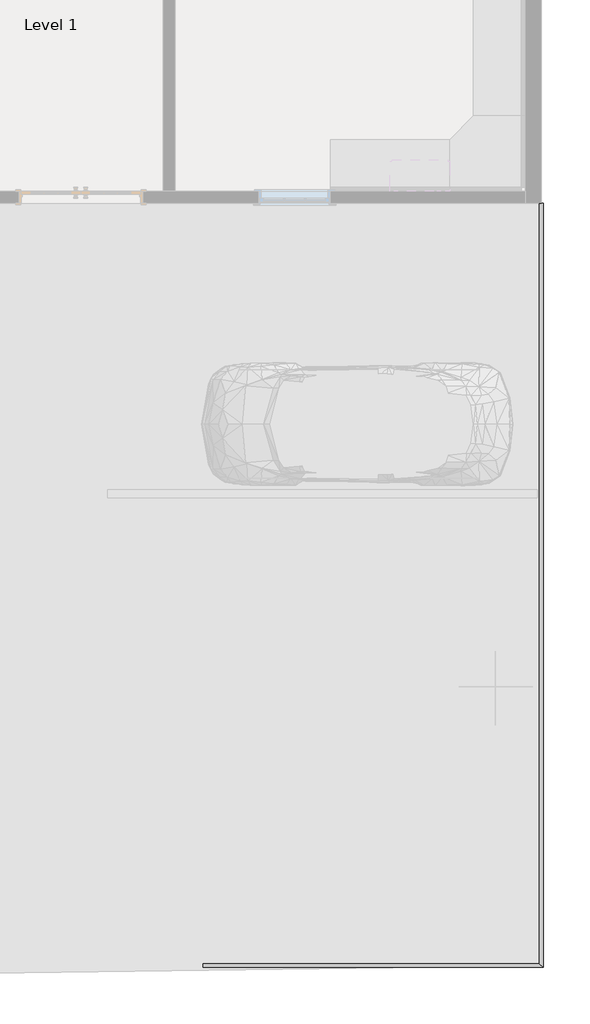
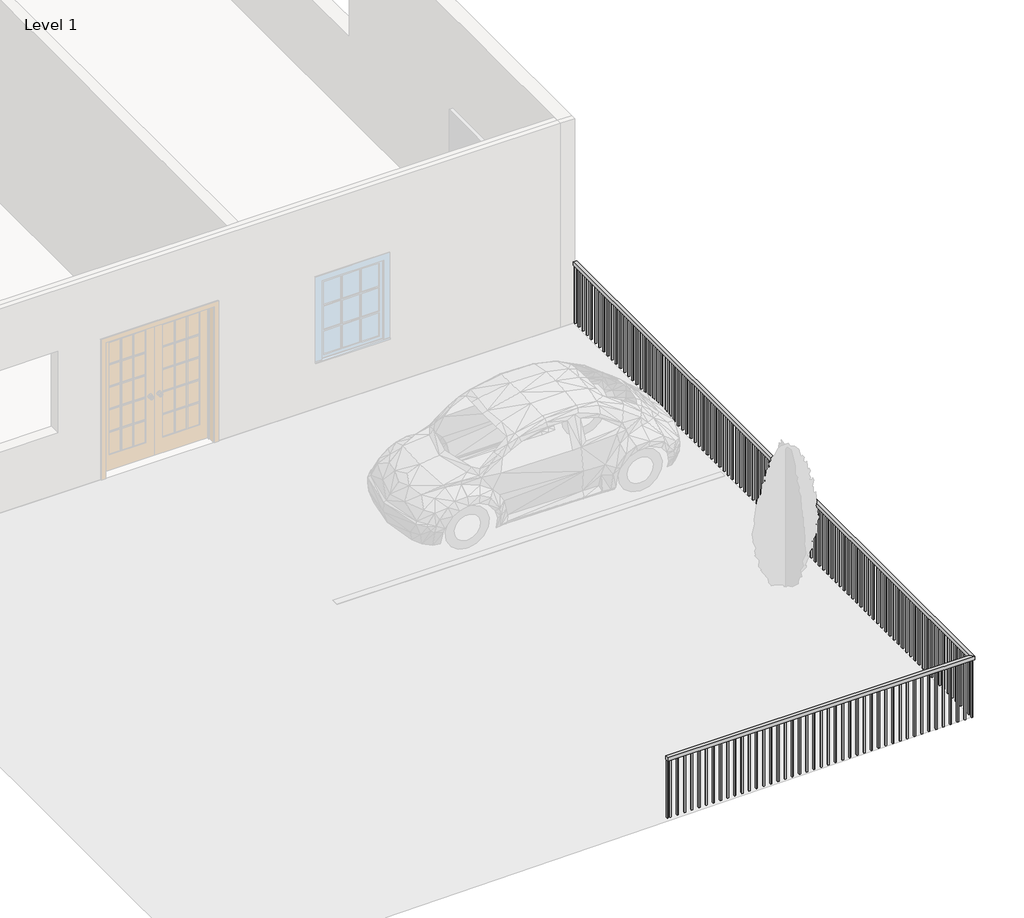
# One storey, part 3 of 5: 1 railing.
"""IFC4 building model written with IfcOpenShell, lengths in millimetres."""

from ifc_helpers import new_model, si_unit, origin, origin_with_axes, place, context, project, spatial, polyline, outline, extrude, faceted_brep, element, save

model = new_model("IFC4")

# Units and contexts
model_context = context("Model", 3, world=origin())
ifc_project = project(units=[si_unit("LENGTHUNIT", "METRE", prefix="MILLI")], contexts=[model_context])

# Site, building, storey
site = spatial("IfcSite", under=ifc_project)
building = spatial("IfcBuilding", under=site)
storey = spatial("IfcBuildingStorey", under=building, Name="Level 1", Elevation=0.0)

# Railing
placement = place(None, origin())
element("IfcRailing", 1, ObjectType="Handrail - Rectangular", at=placement, inside=storey, context=model_context, shape_type="SolidModel", body=[
    faceted_brep([(1884.1829734, -2473.4076646, 914.4), (1884.1829734, -2473.4076646, 863.6), (1833.3829734, -2473.4076646, 863.6), (1833.3829734, -2473.4076646, 914.4), (1884.1829734, -12227.0076646, 914.4), (1884.1829734, -12227.0076646, 863.6), (1833.3829734, -12176.2076646, 863.6), (1833.3829734, -12176.2076646, 914.4), (-2459.2170266, -12227.0076646, 914.4), (-2459.2170266, -12176.2076646, 914.4), (-2459.2170266, -12176.2076646, 863.6), (-2459.2170266, -12227.0076646, 863.6)], [[[0, 1, 2, 3]], [[1, 0, 4, 5]], [[2, 1, 5, 6]], [[3, 2, 6, 7]], [[0, 3, 7, 4]], [[8, 9, 10, 11]], [[5, 4, 8, 11]], [[6, 5, 11, 10]], [[7, 6, 10, 9]], [[4, 7, 9, 8]]]),
    extrude(outline(polyline([(-2398.8920266, -12192.0826646), (-2398.8920266, -12211.1326646), (-2417.9420266, -12211.1326646), (-2417.9420266, -12192.0826646), (-2398.8920266, -12192.0826646)])), origin_with_axes(), (0.0, 0.0, 1.0), 863.6),
    extrude(outline(polyline([(-2297.2920266, -12192.0826646), (-2297.2920266, -12211.1326646), (-2316.3420266, -12211.1326646), (-2316.3420266, -12192.0826646), (-2297.2920266, -12192.0826646)])), origin_with_axes(), (0.0, 0.0, 1.0), 863.6),
    extrude(outline(polyline([(-2195.6920266, -12192.0826646), (-2195.6920266, -12211.1326646), (-2214.7420266, -12211.1326646), (-2214.7420266, -12192.0826646), (-2195.6920266, -12192.0826646)])), origin_with_axes(), (0.0, 0.0, 1.0), 863.6),
    extrude(outline(polyline([(-2094.0920266, -12192.0826646), (-2094.0920266, -12211.1326646), (-2113.1420266, -12211.1326646), (-2113.1420266, -12192.0826646), (-2094.0920266, -12192.0826646)])), origin_with_axes(), (0.0, 0.0, 1.0), 863.6),
    extrude(outline(polyline([(-1992.4920266, -12192.0826646), (-1992.4920266, -12211.1326646), (-2011.5420266, -12211.1326646), (-2011.5420266, -12192.0826646), (-1992.4920266, -12192.0826646)])), origin_with_axes(), (0.0, 0.0, 1.0), 863.6),
    extrude(outline(polyline([(-1890.8920266, -12192.0826646), (-1890.8920266, -12211.1326646), (-1909.9420266, -12211.1326646), (-1909.9420266, -12192.0826646), (-1890.8920266, -12192.0826646)])), origin_with_axes(), (0.0, 0.0, 1.0), 863.6),
    extrude(outline(polyline([(-1789.2920266, -12192.0826646), (-1789.2920266, -12211.1326646), (-1808.3420266, -12211.1326646), (-1808.3420266, -12192.0826646), (-1789.2920266, -12192.0826646)])), origin_with_axes(), (0.0, 0.0, 1.0), 863.6),
    extrude(outline(polyline([(-1687.6920266, -12192.0826646), (-1687.6920266, -12211.1326646), (-1706.7420266, -12211.1326646), (-1706.7420266, -12192.0826646), (-1687.6920266, -12192.0826646)])), origin_with_axes(), (0.0, 0.0, 1.0), 863.6),
    extrude(outline(polyline([(-1586.0920266, -12192.0826646), (-1586.0920266, -12211.1326646), (-1605.1420266, -12211.1326646), (-1605.1420266, -12192.0826646), (-1586.0920266, -12192.0826646)])), origin_with_axes(), (0.0, 0.0, 1.0), 863.6),
    extrude(outline(polyline([(-1484.4920266, -12192.0826646), (-1484.4920266, -12211.1326646), (-1503.5420266, -12211.1326646), (-1503.5420266, -12192.0826646), (-1484.4920266, -12192.0826646)])), origin_with_axes(), (0.0, 0.0, 1.0), 863.6),
    extrude(outline(polyline([(-1382.8920266, -12192.0826646), (-1382.8920266, -12211.1326646), (-1401.9420266, -12211.1326646), (-1401.9420266, -12192.0826646), (-1382.8920266, -12192.0826646)])), origin_with_axes(), (0.0, 0.0, 1.0), 863.6),
    extrude(outline(polyline([(-1281.2920266, -12192.0826646), (-1281.2920266, -12211.1326646), (-1300.3420266, -12211.1326646), (-1300.3420266, -12192.0826646), (-1281.2920266, -12192.0826646)])), origin_with_axes(), (0.0, 0.0, 1.0), 863.6),
    extrude(outline(polyline([(-1179.6920266, -12192.0826646), (-1179.6920266, -12211.1326646), (-1198.7420266, -12211.1326646), (-1198.7420266, -12192.0826646), (-1179.6920266, -12192.0826646)])), origin_with_axes(), (0.0, 0.0, 1.0), 863.6),
    extrude(outline(polyline([(-1078.0920266, -12192.0826646), (-1078.0920266, -12211.1326646), (-1097.1420266, -12211.1326646), (-1097.1420266, -12192.0826646), (-1078.0920266, -12192.0826646)])), origin_with_axes(), (0.0, 0.0, 1.0), 863.6),
    extrude(outline(polyline([(-976.4920266, -12192.0826646), (-976.4920266, -12211.1326646), (-995.5420266, -12211.1326646), (-995.5420266, -12192.0826646), (-976.4920266, -12192.0826646)])), origin_with_axes(), (0.0, 0.0, 1.0), 863.6),
    extrude(outline(polyline([(-874.8920266, -12192.0826646), (-874.8920266, -12211.1326646), (-893.9420266, -12211.1326646), (-893.9420266, -12192.0826646), (-874.8920266, -12192.0826646)])), origin_with_axes(), (0.0, 0.0, 1.0), 863.6),
    extrude(outline(polyline([(-773.2920266, -12192.0826646), (-773.2920266, -12211.1326646), (-792.3420266, -12211.1326646), (-792.3420266, -12192.0826646), (-773.2920266, -12192.0826646)])), origin_with_axes(), (0.0, 0.0, 1.0), 863.6),
    extrude(outline(polyline([(-671.6920266, -12192.0826646), (-671.6920266, -12211.1326646), (-690.7420266, -12211.1326646), (-690.7420266, -12192.0826646), (-671.6920266, -12192.0826646)])), origin_with_axes(), (0.0, 0.0, 1.0), 863.6),
    extrude(outline(polyline([(-570.0920266, -12192.0826646), (-570.0920266, -12211.1326646), (-589.1420266, -12211.1326646), (-589.1420266, -12192.0826646), (-570.0920266, -12192.0826646)])), origin_with_axes(), (0.0, 0.0, 1.0), 863.6),
    extrude(outline(polyline([(-468.4920266, -12192.0826646), (-468.4920266, -12211.1326646), (-487.5420266, -12211.1326646), (-487.5420266, -12192.0826646), (-468.4920266, -12192.0826646)])), origin_with_axes(), (0.0, 0.0, 1.0), 863.6),
    extrude(outline(polyline([(-366.8920266, -12192.0826646), (-366.8920266, -12211.1326646), (-385.9420266, -12211.1326646), (-385.9420266, -12192.0826646), (-366.8920266, -12192.0826646)])), origin_with_axes(), (0.0, 0.0, 1.0), 863.6),
    extrude(outline(polyline([(-265.2920266, -12192.0826646), (-265.2920266, -12211.1326646), (-284.3420266, -12211.1326646), (-284.3420266, -12192.0826646), (-265.2920266, -12192.0826646)])), origin_with_axes(), (0.0, 0.0, 1.0), 863.6),
    extrude(outline(polyline([(-163.6920266, -12192.0826646), (-163.6920266, -12211.1326646), (-182.7420266, -12211.1326646), (-182.7420266, -12192.0826646), (-163.6920266, -12192.0826646)])), origin_with_axes(), (0.0, 0.0, 1.0), 863.6),
    extrude(outline(polyline([(-62.0920266, -12192.0826646), (-62.0920266, -12211.1326646), (-81.1420266, -12211.1326646), (-81.1420266, -12192.0826646), (-62.0920266, -12192.0826646)])), origin_with_axes(), (0.0, 0.0, 1.0), 863.6),
    extrude(outline(polyline([(39.5079734, -12192.0826646), (39.5079734, -12211.1326646), (20.4579734, -12211.1326646), (20.4579734, -12192.0826646), (39.5079734, -12192.0826646)])), origin_with_axes(), (0.0, 0.0, 1.0), 863.6),
    extrude(outline(polyline([(141.1079734, -12192.0826646), (141.1079734, -12211.1326646), (122.0579734, -12211.1326646), (122.0579734, -12192.0826646), (141.1079734, -12192.0826646)])), origin_with_axes(), (0.0, 0.0, 1.0), 863.6),
    extrude(outline(polyline([(242.7079734, -12192.0826646), (242.7079734, -12211.1326646), (223.6579734, -12211.1326646), (223.6579734, -12192.0826646), (242.7079734, -12192.0826646)])), origin_with_axes(), (0.0, 0.0, 1.0), 863.6),
    extrude(outline(polyline([(344.3079734, -12192.0826646), (344.3079734, -12211.1326646), (325.2579734, -12211.1326646), (325.2579734, -12192.0826646), (344.3079734, -12192.0826646)])), origin_with_axes(), (0.0, 0.0, 1.0), 863.6),
    extrude(outline(polyline([(445.9079734, -12192.0826646), (445.9079734, -12211.1326646), (426.8579734, -12211.1326646), (426.8579734, -12192.0826646), (445.9079734, -12192.0826646)])), origin_with_axes(), (0.0, 0.0, 1.0), 863.6),
    extrude(outline(polyline([(547.5079734, -12192.0826646), (547.5079734, -12211.1326646), (528.4579734, -12211.1326646), (528.4579734, -12192.0826646), (547.5079734, -12192.0826646)])), origin_with_axes(), (0.0, 0.0, 1.0), 863.6),
    extrude(outline(polyline([(649.1079734, -12192.0826646), (649.1079734, -12211.1326646), (630.0579734, -12211.1326646), (630.0579734, -12192.0826646), (649.1079734, -12192.0826646)])), origin_with_axes(), (0.0, 0.0, 1.0), 863.6),
    extrude(outline(polyline([(750.7079734, -12192.0826646), (750.7079734, -12211.1326646), (731.6579734, -12211.1326646), (731.6579734, -12192.0826646), (750.7079734, -12192.0826646)])), origin_with_axes(), (0.0, 0.0, 1.0), 863.6),
    extrude(outline(polyline([(852.3079734, -12192.0826646), (852.3079734, -12211.1326646), (833.2579734, -12211.1326646), (833.2579734, -12192.0826646), (852.3079734, -12192.0826646)])), origin_with_axes(), (0.0, 0.0, 1.0), 863.6),
    extrude(outline(polyline([(953.9079734, -12192.0826646), (953.9079734, -12211.1326646), (934.8579734, -12211.1326646), (934.8579734, -12192.0826646), (953.9079734, -12192.0826646)])), origin_with_axes(), (0.0, 0.0, 1.0), 863.6),
    extrude(outline(polyline([(1055.5079734, -12192.0826646), (1055.5079734, -12211.1326646), (1036.4579734, -12211.1326646), (1036.4579734, -12192.0826646), (1055.5079734, -12192.0826646)])), origin_with_axes(), (0.0, 0.0, 1.0), 863.6),
    extrude(outline(polyline([(1157.1079734, -12192.0826646), (1157.1079734, -12211.1326646), (1138.0579734, -12211.1326646), (1138.0579734, -12192.0826646), (1157.1079734, -12192.0826646)])), origin_with_axes(), (0.0, 0.0, 1.0), 863.6),
    extrude(outline(polyline([(1258.7079734, -12192.0826646), (1258.7079734, -12211.1326646), (1239.6579734, -12211.1326646), (1239.6579734, -12192.0826646), (1258.7079734, -12192.0826646)])), origin_with_axes(), (0.0, 0.0, 1.0), 863.6),
    extrude(outline(polyline([(1360.3079734, -12192.0826646), (1360.3079734, -12211.1326646), (1341.2579734, -12211.1326646), (1341.2579734, -12192.0826646), (1360.3079734, -12192.0826646)])), origin_with_axes(), (0.0, 0.0, 1.0), 863.6),
    extrude(outline(polyline([(1461.9079734, -12192.0826646), (1461.9079734, -12211.1326646), (1442.8579734, -12211.1326646), (1442.8579734, -12192.0826646), (1461.9079734, -12192.0826646)])), origin_with_axes(), (0.0, 0.0, 1.0), 863.6),
    extrude(outline(polyline([(1563.5079734, -12192.0826646), (1563.5079734, -12211.1326646), (1544.4579734, -12211.1326646), (1544.4579734, -12192.0826646), (1563.5079734, -12192.0826646)])), origin_with_axes(), (0.0, 0.0, 1.0), 863.6),
    extrude(outline(polyline([(1665.1079734, -12192.0826646), (1665.1079734, -12211.1326646), (1646.0579734, -12211.1326646), (1646.0579734, -12192.0826646), (1665.1079734, -12192.0826646)])), origin_with_axes(), (0.0, 0.0, 1.0), 863.6),
    extrude(outline(polyline([(1766.7079734, -12192.0826646), (1766.7079734, -12211.1326646), (1747.6579734, -12211.1326646), (1747.6579734, -12192.0826646), (1766.7079734, -12192.0826646)])), origin_with_axes(), (0.0, 0.0, 1.0), 863.6),
    extrude(outline(polyline([(1849.2579734, -12115.8826646), (1868.3079734, -12115.8826646), (1868.3079734, -12134.9326646), (1849.2579734, -12134.9326646), (1849.2579734, -12115.8826646)])), origin_with_axes(), (0.0, 0.0, 1.0), 863.6),
    extrude(outline(polyline([(1849.2579734, -12014.2826646), (1868.3079734, -12014.2826646), (1868.3079734, -12033.3326646), (1849.2579734, -12033.3326646), (1849.2579734, -12014.2826646)])), origin_with_axes(), (0.0, 0.0, 1.0), 863.6),
    extrude(outline(polyline([(1849.2579734, -11912.6826646), (1868.3079734, -11912.6826646), (1868.3079734, -11931.7326646), (1849.2579734, -11931.7326646), (1849.2579734, -11912.6826646)])), origin_with_axes(), (0.0, 0.0, 1.0), 863.6),
    extrude(outline(polyline([(1849.2579734, -11811.0826646), (1868.3079734, -11811.0826646), (1868.3079734, -11830.1326646), (1849.2579734, -11830.1326646), (1849.2579734, -11811.0826646)])), origin_with_axes(), (0.0, 0.0, 1.0), 863.6),
    extrude(outline(polyline([(1849.2579734, -11709.4826646), (1868.3079734, -11709.4826646), (1868.3079734, -11728.5326646), (1849.2579734, -11728.5326646), (1849.2579734, -11709.4826646)])), origin_with_axes(), (0.0, 0.0, 1.0), 863.6),
    extrude(outline(polyline([(1849.2579734, -11607.8826646), (1868.3079734, -11607.8826646), (1868.3079734, -11626.9326646), (1849.2579734, -11626.9326646), (1849.2579734, -11607.8826646)])), origin_with_axes(), (0.0, 0.0, 1.0), 863.6),
    extrude(outline(polyline([(1849.2579734, -11506.2826646), (1868.3079734, -11506.2826646), (1868.3079734, -11525.3326646), (1849.2579734, -11525.3326646), (1849.2579734, -11506.2826646)])), origin_with_axes(), (0.0, 0.0, 1.0), 863.6),
    extrude(outline(polyline([(1849.2579734, -11404.6826646), (1868.3079734, -11404.6826646), (1868.3079734, -11423.7326646), (1849.2579734, -11423.7326646), (1849.2579734, -11404.6826646)])), origin_with_axes(), (0.0, 0.0, 1.0), 863.6),
    extrude(outline(polyline([(1849.2579734, -11303.0826646), (1868.3079734, -11303.0826646), (1868.3079734, -11322.1326646), (1849.2579734, -11322.1326646), (1849.2579734, -11303.0826646)])), origin_with_axes(), (0.0, 0.0, 1.0), 863.6),
    extrude(outline(polyline([(1849.2579734, -11201.4826646), (1868.3079734, -11201.4826646), (1868.3079734, -11220.5326646), (1849.2579734, -11220.5326646), (1849.2579734, -11201.4826646)])), origin_with_axes(), (0.0, 0.0, 1.0), 863.6),
    extrude(outline(polyline([(1849.2579734, -11099.8826646), (1868.3079734, -11099.8826646), (1868.3079734, -11118.9326646), (1849.2579734, -11118.9326646), (1849.2579734, -11099.8826646)])), origin_with_axes(), (0.0, 0.0, 1.0), 863.6),
    extrude(outline(polyline([(1849.2579734, -10998.2826646), (1868.3079734, -10998.2826646), (1868.3079734, -11017.3326646), (1849.2579734, -11017.3326646), (1849.2579734, -10998.2826646)])), origin_with_axes(), (0.0, 0.0, 1.0), 863.6),
    extrude(outline(polyline([(1849.2579734, -10896.6826646), (1868.3079734, -10896.6826646), (1868.3079734, -10915.7326646), (1849.2579734, -10915.7326646), (1849.2579734, -10896.6826646)])), origin_with_axes(), (0.0, 0.0, 1.0), 863.6),
    extrude(outline(polyline([(1849.2579734, -10795.0826646), (1868.3079734, -10795.0826646), (1868.3079734, -10814.1326646), (1849.2579734, -10814.1326646), (1849.2579734, -10795.0826646)])), origin_with_axes(), (0.0, 0.0, 1.0), 863.6),
    extrude(outline(polyline([(1849.2579734, -10693.4826646), (1868.3079734, -10693.4826646), (1868.3079734, -10712.5326646), (1849.2579734, -10712.5326646), (1849.2579734, -10693.4826646)])), origin_with_axes(), (0.0, 0.0, 1.0), 863.6),
    extrude(outline(polyline([(1849.2579734, -10591.8826646), (1868.3079734, -10591.8826646), (1868.3079734, -10610.9326646), (1849.2579734, -10610.9326646), (1849.2579734, -10591.8826646)])), origin_with_axes(), (0.0, 0.0, 1.0), 863.6),
    extrude(outline(polyline([(1849.2579734, -10490.2826646), (1868.3079734, -10490.2826646), (1868.3079734, -10509.3326646), (1849.2579734, -10509.3326646), (1849.2579734, -10490.2826646)])), origin_with_axes(), (0.0, 0.0, 1.0), 863.6),
    extrude(outline(polyline([(1849.2579734, -10388.6826646), (1868.3079734, -10388.6826646), (1868.3079734, -10407.7326646), (1849.2579734, -10407.7326646), (1849.2579734, -10388.6826646)])), origin_with_axes(), (0.0, 0.0, 1.0), 863.6),
    extrude(outline(polyline([(1849.2579734, -10287.0826646), (1868.3079734, -10287.0826646), (1868.3079734, -10306.1326646), (1849.2579734, -10306.1326646), (1849.2579734, -10287.0826646)])), origin_with_axes(), (0.0, 0.0, 1.0), 863.6),
    extrude(outline(polyline([(1849.2579734, -10185.4826646), (1868.3079734, -10185.4826646), (1868.3079734, -10204.5326646), (1849.2579734, -10204.5326646), (1849.2579734, -10185.4826646)])), origin_with_axes(), (0.0, 0.0, 1.0), 863.6),
    extrude(outline(polyline([(1849.2579734, -10083.8826646), (1868.3079734, -10083.8826646), (1868.3079734, -10102.9326646), (1849.2579734, -10102.9326646), (1849.2579734, -10083.8826646)])), origin_with_axes(), (0.0, 0.0, 1.0), 863.6),
    extrude(outline(polyline([(1849.2579734, -9982.2826646), (1868.3079734, -9982.2826646), (1868.3079734, -10001.3326646), (1849.2579734, -10001.3326646), (1849.2579734, -9982.2826646)])), origin_with_axes(), (0.0, 0.0, 1.0), 863.6),
    extrude(outline(polyline([(1849.2579734, -9880.6826646), (1868.3079734, -9880.6826646), (1868.3079734, -9899.7326646), (1849.2579734, -9899.7326646), (1849.2579734, -9880.6826646)])), origin_with_axes(), (0.0, 0.0, 1.0), 863.6),
    extrude(outline(polyline([(1849.2579734, -9779.0826646), (1868.3079734, -9779.0826646), (1868.3079734, -9798.1326646), (1849.2579734, -9798.1326646), (1849.2579734, -9779.0826646)])), origin_with_axes(), (0.0, 0.0, 1.0), 863.6),
    extrude(outline(polyline([(1849.2579734, -9677.4826646), (1868.3079734, -9677.4826646), (1868.3079734, -9696.5326646), (1849.2579734, -9696.5326646), (1849.2579734, -9677.4826646)])), origin_with_axes(), (0.0, 0.0, 1.0), 863.6),
    extrude(outline(polyline([(1849.2579734, -9575.8826646), (1868.3079734, -9575.8826646), (1868.3079734, -9594.9326646), (1849.2579734, -9594.9326646), (1849.2579734, -9575.8826646)])), origin_with_axes(), (0.0, 0.0, 1.0), 863.6),
    extrude(outline(polyline([(1849.2579734, -9474.2826646), (1868.3079734, -9474.2826646), (1868.3079734, -9493.3326646), (1849.2579734, -9493.3326646), (1849.2579734, -9474.2826646)])), origin_with_axes(), (0.0, 0.0, 1.0), 863.6),
    extrude(outline(polyline([(1849.2579734, -9372.6826646), (1868.3079734, -9372.6826646), (1868.3079734, -9391.7326646), (1849.2579734, -9391.7326646), (1849.2579734, -9372.6826646)])), origin_with_axes(), (0.0, 0.0, 1.0), 863.6),
    extrude(outline(polyline([(1849.2579734, -9271.0826646), (1868.3079734, -9271.0826646), (1868.3079734, -9290.1326646), (1849.2579734, -9290.1326646), (1849.2579734, -9271.0826646)])), origin_with_axes(), (0.0, 0.0, 1.0), 863.6),
    extrude(outline(polyline([(1849.2579734, -9169.4826646), (1868.3079734, -9169.4826646), (1868.3079734, -9188.5326646), (1849.2579734, -9188.5326646), (1849.2579734, -9169.4826646)])), origin_with_axes(), (0.0, 0.0, 1.0), 863.6),
    extrude(outline(polyline([(1849.2579734, -9067.8826646), (1868.3079734, -9067.8826646), (1868.3079734, -9086.9326646), (1849.2579734, -9086.9326646), (1849.2579734, -9067.8826646)])), origin_with_axes(), (0.0, 0.0, 1.0), 863.6),
    extrude(outline(polyline([(1849.2579734, -8966.2826646), (1868.3079734, -8966.2826646), (1868.3079734, -8985.3326646), (1849.2579734, -8985.3326646), (1849.2579734, -8966.2826646)])), origin_with_axes(), (0.0, 0.0, 1.0), 863.6),
    extrude(outline(polyline([(1849.2579734, -8864.6826646), (1868.3079734, -8864.6826646), (1868.3079734, -8883.7326646), (1849.2579734, -8883.7326646), (1849.2579734, -8864.6826646)])), origin_with_axes(), (0.0, 0.0, 1.0), 863.6),
    extrude(outline(polyline([(1849.2579734, -8763.0826646), (1868.3079734, -8763.0826646), (1868.3079734, -8782.1326646), (1849.2579734, -8782.1326646), (1849.2579734, -8763.0826646)])), origin_with_axes(), (0.0, 0.0, 1.0), 863.6),
    extrude(outline(polyline([(1849.2579734, -8661.4826646), (1868.3079734, -8661.4826646), (1868.3079734, -8680.5326646), (1849.2579734, -8680.5326646), (1849.2579734, -8661.4826646)])), origin_with_axes(), (0.0, 0.0, 1.0), 863.6),
    extrude(outline(polyline([(1849.2579734, -8559.8826646), (1868.3079734, -8559.8826646), (1868.3079734, -8578.9326646), (1849.2579734, -8578.9326646), (1849.2579734, -8559.8826646)])), origin_with_axes(), (0.0, 0.0, 1.0), 863.6),
    extrude(outline(polyline([(1849.2579734, -8458.2826646), (1868.3079734, -8458.2826646), (1868.3079734, -8477.3326646), (1849.2579734, -8477.3326646), (1849.2579734, -8458.2826646)])), origin_with_axes(), (0.0, 0.0, 1.0), 863.6),
    extrude(outline(polyline([(1849.2579734, -8356.6826646), (1868.3079734, -8356.6826646), (1868.3079734, -8375.7326646), (1849.2579734, -8375.7326646), (1849.2579734, -8356.6826646)])), origin_with_axes(), (0.0, 0.0, 1.0), 863.6),
    extrude(outline(polyline([(1849.2579734, -8255.0826646), (1868.3079734, -8255.0826646), (1868.3079734, -8274.1326646), (1849.2579734, -8274.1326646), (1849.2579734, -8255.0826646)])), origin_with_axes(), (0.0, 0.0, 1.0), 863.6),
    extrude(outline(polyline([(1849.2579734, -8153.4826646), (1868.3079734, -8153.4826646), (1868.3079734, -8172.5326646), (1849.2579734, -8172.5326646), (1849.2579734, -8153.4826646)])), origin_with_axes(), (0.0, 0.0, 1.0), 863.6),
    extrude(outline(polyline([(1849.2579734, -8051.8826646), (1868.3079734, -8051.8826646), (1868.3079734, -8070.9326646), (1849.2579734, -8070.9326646), (1849.2579734, -8051.8826646)])), origin_with_axes(), (0.0, 0.0, 1.0), 863.6),
    extrude(outline(polyline([(1849.2579734, -7950.2826646), (1868.3079734, -7950.2826646), (1868.3079734, -7969.3326646), (1849.2579734, -7969.3326646), (1849.2579734, -7950.2826646)])), origin_with_axes(), (0.0, 0.0, 1.0), 863.6),
    extrude(outline(polyline([(1849.2579734, -7848.6826646), (1868.3079734, -7848.6826646), (1868.3079734, -7867.7326646), (1849.2579734, -7867.7326646), (1849.2579734, -7848.6826646)])), origin_with_axes(), (0.0, 0.0, 1.0), 863.6),
    extrude(outline(polyline([(1849.2579734, -7747.0826646), (1868.3079734, -7747.0826646), (1868.3079734, -7766.1326646), (1849.2579734, -7766.1326646), (1849.2579734, -7747.0826646)])), origin_with_axes(), (0.0, 0.0, 1.0), 863.6),
    extrude(outline(polyline([(1849.2579734, -7645.4826646), (1868.3079734, -7645.4826646), (1868.3079734, -7664.5326646), (1849.2579734, -7664.5326646), (1849.2579734, -7645.4826646)])), origin_with_axes(), (0.0, 0.0, 1.0), 863.6),
    extrude(outline(polyline([(1849.2579734, -7543.8826646), (1868.3079734, -7543.8826646), (1868.3079734, -7562.9326646), (1849.2579734, -7562.9326646), (1849.2579734, -7543.8826646)])), origin_with_axes(), (0.0, 0.0, 1.0), 863.6),
    extrude(outline(polyline([(1849.2579734, -7442.2826646), (1868.3079734, -7442.2826646), (1868.3079734, -7461.3326646), (1849.2579734, -7461.3326646), (1849.2579734, -7442.2826646)])), origin_with_axes(), (0.0, 0.0, 1.0), 863.6),
    extrude(outline(polyline([(1849.2579734, -7340.6826646), (1868.3079734, -7340.6826646), (1868.3079734, -7359.7326646), (1849.2579734, -7359.7326646), (1849.2579734, -7340.6826646)])), origin_with_axes(), (0.0, 0.0, 1.0), 863.6),
    extrude(outline(polyline([(1849.2579734, -7239.0826646), (1868.3079734, -7239.0826646), (1868.3079734, -7258.1326646), (1849.2579734, -7258.1326646), (1849.2579734, -7239.0826646)])), origin_with_axes(), (0.0, 0.0, 1.0), 863.6),
    extrude(outline(polyline([(1849.2579734, -7137.4826646), (1868.3079734, -7137.4826646), (1868.3079734, -7156.5326646), (1849.2579734, -7156.5326646), (1849.2579734, -7137.4826646)])), origin_with_axes(), (0.0, 0.0, 1.0), 863.6),
    extrude(outline(polyline([(1849.2579734, -7035.8826646), (1868.3079734, -7035.8826646), (1868.3079734, -7054.9326646), (1849.2579734, -7054.9326646), (1849.2579734, -7035.8826646)])), origin_with_axes(), (0.0, 0.0, 1.0), 863.6),
    extrude(outline(polyline([(1849.2579734, -6934.2826646), (1868.3079734, -6934.2826646), (1868.3079734, -6953.3326646), (1849.2579734, -6953.3326646), (1849.2579734, -6934.2826646)])), origin_with_axes(), (0.0, 0.0, 1.0), 863.6),
    extrude(outline(polyline([(1849.2579734, -6832.6826646), (1868.3079734, -6832.6826646), (1868.3079734, -6851.7326646), (1849.2579734, -6851.7326646), (1849.2579734, -6832.6826646)])), origin_with_axes(), (0.0, 0.0, 1.0), 863.6),
    extrude(outline(polyline([(1849.2579734, -6731.0826646), (1868.3079734, -6731.0826646), (1868.3079734, -6750.1326646), (1849.2579734, -6750.1326646), (1849.2579734, -6731.0826646)])), origin_with_axes(), (0.0, 0.0, 1.0), 863.6),
    extrude(outline(polyline([(1849.2579734, -6629.4826646), (1868.3079734, -6629.4826646), (1868.3079734, -6648.5326646), (1849.2579734, -6648.5326646), (1849.2579734, -6629.4826646)])), origin_with_axes(), (0.0, 0.0, 1.0), 863.6),
    extrude(outline(polyline([(1849.2579734, -6527.8826646), (1868.3079734, -6527.8826646), (1868.3079734, -6546.9326646), (1849.2579734, -6546.9326646), (1849.2579734, -6527.8826646)])), origin_with_axes(), (0.0, 0.0, 1.0), 863.6),
    extrude(outline(polyline([(1849.2579734, -6426.2826646), (1868.3079734, -6426.2826646), (1868.3079734, -6445.3326646), (1849.2579734, -6445.3326646), (1849.2579734, -6426.2826646)])), origin_with_axes(), (0.0, 0.0, 1.0), 863.6),
    extrude(outline(polyline([(1849.2579734, -6324.6826646), (1868.3079734, -6324.6826646), (1868.3079734, -6343.7326646), (1849.2579734, -6343.7326646), (1849.2579734, -6324.6826646)])), origin_with_axes(), (0.0, 0.0, 1.0), 863.6),
    extrude(outline(polyline([(1849.2579734, -6223.0826646), (1868.3079734, -6223.0826646), (1868.3079734, -6242.1326646), (1849.2579734, -6242.1326646), (1849.2579734, -6223.0826646)])), origin_with_axes(), (0.0, 0.0, 1.0), 863.6),
    extrude(outline(polyline([(1849.2579734, -6121.4826646), (1868.3079734, -6121.4826646), (1868.3079734, -6140.5326646), (1849.2579734, -6140.5326646), (1849.2579734, -6121.4826646)])), origin_with_axes(), (0.0, 0.0, 1.0), 863.6),
    extrude(outline(polyline([(1849.2579734, -6019.8826646), (1868.3079734, -6019.8826646), (1868.3079734, -6038.9326646), (1849.2579734, -6038.9326646), (1849.2579734, -6019.8826646)])), origin_with_axes(), (0.0, 0.0, 1.0), 863.6),
    extrude(outline(polyline([(1849.2579734, -5918.2826646), (1868.3079734, -5918.2826646), (1868.3079734, -5937.3326646), (1849.2579734, -5937.3326646), (1849.2579734, -5918.2826646)])), origin_with_axes(), (0.0, 0.0, 1.0), 863.6),
    extrude(outline(polyline([(1849.2579734, -5816.6826646), (1868.3079734, -5816.6826646), (1868.3079734, -5835.7326646), (1849.2579734, -5835.7326646), (1849.2579734, -5816.6826646)])), origin_with_axes(), (0.0, 0.0, 1.0), 863.6),
    extrude(outline(polyline([(1849.2579734, -5715.0826646), (1868.3079734, -5715.0826646), (1868.3079734, -5734.1326646), (1849.2579734, -5734.1326646), (1849.2579734, -5715.0826646)])), origin_with_axes(), (0.0, 0.0, 1.0), 863.6),
    extrude(outline(polyline([(1849.2579734, -5613.4826646), (1868.3079734, -5613.4826646), (1868.3079734, -5632.5326646), (1849.2579734, -5632.5326646), (1849.2579734, -5613.4826646)])), origin_with_axes(), (0.0, 0.0, 1.0), 863.6),
    extrude(outline(polyline([(1849.2579734, -5511.8826646), (1868.3079734, -5511.8826646), (1868.3079734, -5530.9326646), (1849.2579734, -5530.9326646), (1849.2579734, -5511.8826646)])), origin_with_axes(), (0.0, 0.0, 1.0), 863.6),
    extrude(outline(polyline([(1849.2579734, -5410.2826646), (1868.3079734, -5410.2826646), (1868.3079734, -5429.3326646), (1849.2579734, -5429.3326646), (1849.2579734, -5410.2826646)])), origin_with_axes(), (0.0, 0.0, 1.0), 863.6),
    extrude(outline(polyline([(1849.2579734, -5308.6826646), (1868.3079734, -5308.6826646), (1868.3079734, -5327.7326646), (1849.2579734, -5327.7326646), (1849.2579734, -5308.6826646)])), origin_with_axes(), (0.0, 0.0, 1.0), 863.6),
    extrude(outline(polyline([(1849.2579734, -5207.0826646), (1868.3079734, -5207.0826646), (1868.3079734, -5226.1326646), (1849.2579734, -5226.1326646), (1849.2579734, -5207.0826646)])), origin_with_axes(), (0.0, 0.0, 1.0), 863.6),
    extrude(outline(polyline([(1849.2579734, -5105.4826646), (1868.3079734, -5105.4826646), (1868.3079734, -5124.5326646), (1849.2579734, -5124.5326646), (1849.2579734, -5105.4826646)])), origin_with_axes(), (0.0, 0.0, 1.0), 863.6),
    extrude(outline(polyline([(1849.2579734, -5003.8826646), (1868.3079734, -5003.8826646), (1868.3079734, -5022.9326646), (1849.2579734, -5022.9326646), (1849.2579734, -5003.8826646)])), origin_with_axes(), (0.0, 0.0, 1.0), 863.6),
    extrude(outline(polyline([(1849.2579734, -4902.2826646), (1868.3079734, -4902.2826646), (1868.3079734, -4921.3326646), (1849.2579734, -4921.3326646), (1849.2579734, -4902.2826646)])), origin_with_axes(), (0.0, 0.0, 1.0), 863.6),
    extrude(outline(polyline([(1849.2579734, -4800.6826646), (1868.3079734, -4800.6826646), (1868.3079734, -4819.7326646), (1849.2579734, -4819.7326646), (1849.2579734, -4800.6826646)])), origin_with_axes(), (0.0, 0.0, 1.0), 863.6),
    extrude(outline(polyline([(1849.2579734, -4699.0826646), (1868.3079734, -4699.0826646), (1868.3079734, -4718.1326646), (1849.2579734, -4718.1326646), (1849.2579734, -4699.0826646)])), origin_with_axes(), (0.0, 0.0, 1.0), 863.6),
    extrude(outline(polyline([(1849.2579734, -4597.4826646), (1868.3079734, -4597.4826646), (1868.3079734, -4616.5326646), (1849.2579734, -4616.5326646), (1849.2579734, -4597.4826646)])), origin_with_axes(), (0.0, 0.0, 1.0), 863.6),
    extrude(outline(polyline([(1849.2579734, -4495.8826646), (1868.3079734, -4495.8826646), (1868.3079734, -4514.9326646), (1849.2579734, -4514.9326646), (1849.2579734, -4495.8826646)])), origin_with_axes(), (0.0, 0.0, 1.0), 863.6),
    extrude(outline(polyline([(1849.2579734, -4394.2826646), (1868.3079734, -4394.2826646), (1868.3079734, -4413.3326646), (1849.2579734, -4413.3326646), (1849.2579734, -4394.2826646)])), origin_with_axes(), (0.0, 0.0, 1.0), 863.6),
    extrude(outline(polyline([(1849.2579734, -4292.6826646), (1868.3079734, -4292.6826646), (1868.3079734, -4311.7326646), (1849.2579734, -4311.7326646), (1849.2579734, -4292.6826646)])), origin_with_axes(), (0.0, 0.0, 1.0), 863.6),
    extrude(outline(polyline([(1849.2579734, -4191.0826646), (1868.3079734, -4191.0826646), (1868.3079734, -4210.1326646), (1849.2579734, -4210.1326646), (1849.2579734, -4191.0826646)])), origin_with_axes(), (0.0, 0.0, 1.0), 863.6),
    extrude(outline(polyline([(1849.2579734, -4089.4826646), (1868.3079734, -4089.4826646), (1868.3079734, -4108.5326646), (1849.2579734, -4108.5326646), (1849.2579734, -4089.4826646)])), origin_with_axes(), (0.0, 0.0, 1.0), 863.6),
    extrude(outline(polyline([(1849.2579734, -3987.8826646), (1868.3079734, -3987.8826646), (1868.3079734, -4006.9326646), (1849.2579734, -4006.9326646), (1849.2579734, -3987.8826646)])), origin_with_axes(), (0.0, 0.0, 1.0), 863.6),
    extrude(outline(polyline([(1849.2579734, -3886.2826646), (1868.3079734, -3886.2826646), (1868.3079734, -3905.3326646), (1849.2579734, -3905.3326646), (1849.2579734, -3886.2826646)])), origin_with_axes(), (0.0, 0.0, 1.0), 863.6),
    extrude(outline(polyline([(1849.2579734, -3784.6826646), (1868.3079734, -3784.6826646), (1868.3079734, -3803.7326646), (1849.2579734, -3803.7326646), (1849.2579734, -3784.6826646)])), origin_with_axes(), (0.0, 0.0, 1.0), 863.6),
    extrude(outline(polyline([(1849.2579734, -3683.0826646), (1868.3079734, -3683.0826646), (1868.3079734, -3702.1326646), (1849.2579734, -3702.1326646), (1849.2579734, -3683.0826646)])), origin_with_axes(), (0.0, 0.0, 1.0), 863.6),
    extrude(outline(polyline([(1849.2579734, -3581.4826646), (1868.3079734, -3581.4826646), (1868.3079734, -3600.5326646), (1849.2579734, -3600.5326646), (1849.2579734, -3581.4826646)])), origin_with_axes(), (0.0, 0.0, 1.0), 863.6),
    extrude(outline(polyline([(1849.2579734, -3479.8826646), (1868.3079734, -3479.8826646), (1868.3079734, -3498.9326646), (1849.2579734, -3498.9326646), (1849.2579734, -3479.8826646)])), origin_with_axes(), (0.0, 0.0, 1.0), 863.6),
    extrude(outline(polyline([(1849.2579734, -3378.2826646), (1868.3079734, -3378.2826646), (1868.3079734, -3397.3326646), (1849.2579734, -3397.3326646), (1849.2579734, -3378.2826646)])), origin_with_axes(), (0.0, 0.0, 1.0), 863.6),
    extrude(outline(polyline([(1849.2579734, -3276.6826646), (1868.3079734, -3276.6826646), (1868.3079734, -3295.7326646), (1849.2579734, -3295.7326646), (1849.2579734, -3276.6826646)])), origin_with_axes(), (0.0, 0.0, 1.0), 863.6),
    extrude(outline(polyline([(1849.2579734, -3175.0826646), (1868.3079734, -3175.0826646), (1868.3079734, -3194.1326646), (1849.2579734, -3194.1326646), (1849.2579734, -3175.0826646)])), origin_with_axes(), (0.0, 0.0, 1.0), 863.6),
    extrude(outline(polyline([(1849.2579734, -3073.4826646), (1868.3079734, -3073.4826646), (1868.3079734, -3092.5326646), (1849.2579734, -3092.5326646), (1849.2579734, -3073.4826646)])), origin_with_axes(), (0.0, 0.0, 1.0), 863.6),
    extrude(outline(polyline([(1849.2579734, -2971.8826646), (1868.3079734, -2971.8826646), (1868.3079734, -2990.9326646), (1849.2579734, -2990.9326646), (1849.2579734, -2971.8826646)])), origin_with_axes(), (0.0, 0.0, 1.0), 863.6),
    extrude(outline(polyline([(1849.2579734, -2870.2826646), (1868.3079734, -2870.2826646), (1868.3079734, -2889.3326646), (1849.2579734, -2889.3326646), (1849.2579734, -2870.2826646)])), origin_with_axes(), (0.0, 0.0, 1.0), 863.6),
    extrude(outline(polyline([(1849.2579734, -2768.6826646), (1868.3079734, -2768.6826646), (1868.3079734, -2787.7326646), (1849.2579734, -2787.7326646), (1849.2579734, -2768.6826646)])), origin_with_axes(), (0.0, 0.0, 1.0), 863.6),
    extrude(outline(polyline([(1849.2579734, -2667.0826646), (1868.3079734, -2667.0826646), (1868.3079734, -2686.1326646), (1849.2579734, -2686.1326646), (1849.2579734, -2667.0826646)])), origin_with_axes(), (0.0, 0.0, 1.0), 863.6),
    extrude(outline(polyline([(1849.2579734, -2565.4826646), (1868.3079734, -2565.4826646), (1868.3079734, -2584.5326646), (1849.2579734, -2584.5326646), (1849.2579734, -2565.4826646)])), origin_with_axes(), (0.0, 0.0, 1.0), 863.6),
    extrude(outline(polyline([(1849.2579734, -12192.0826646), (1868.3079734, -12192.0826646), (1868.3079734, -12211.1326646), (1849.2579734, -12211.1326646), (1849.2579734, -12192.0826646)])), origin_with_axes(), (0.0, 0.0, 1.0), 863.6),
    extrude(outline(polyline([(-2440.1670266, -12192.0826646), (-2440.1670266, -12211.1326646), (-2459.2170266, -12211.1326646), (-2459.2170266, -12192.0826646), (-2440.1670266, -12192.0826646)])), origin_with_axes(), (0.0, 0.0, 1.0), 863.6),
    extrude(outline(polyline([(1849.2579734, -2473.4076646), (1868.3079734, -2473.4076646), (1868.3079734, -2492.4576646), (1849.2579734, -2492.4576646), (1849.2579734, -2473.4076646)])), origin_with_axes(), (0.0, 0.0, 1.0), 863.6),
])

save(model, "model.ifc")

# Revit data of these elements
# Type "Handrail - Rectangular"
#   Assembly Code = "C2010400"
#   built-in parameter 1008612 = 0.0416667 (stored number, unit not read)
#   built-in parameter 1008611 = 0.0416667 (stored number, unit not read)
#   built-in parameter 1008609 = 0.333333 (stored number, unit not read)
#   built-in parameter 1008604 = 0.166667 (stored number, unit not read)
#   built-in parameter 1008603 = 0.166667 (stored number, unit not read)
#   Railing Height = 3' - 0"
#   built-in parameter 1008630 = 2
#   built-in parameter 1008610 = 2
#   built-in parameter 1008618 = Baluster - Square : 3/4"
# Element 1 (IfcRailing, "Handrail - Rectangular")
#   Phase Created = New Construction
